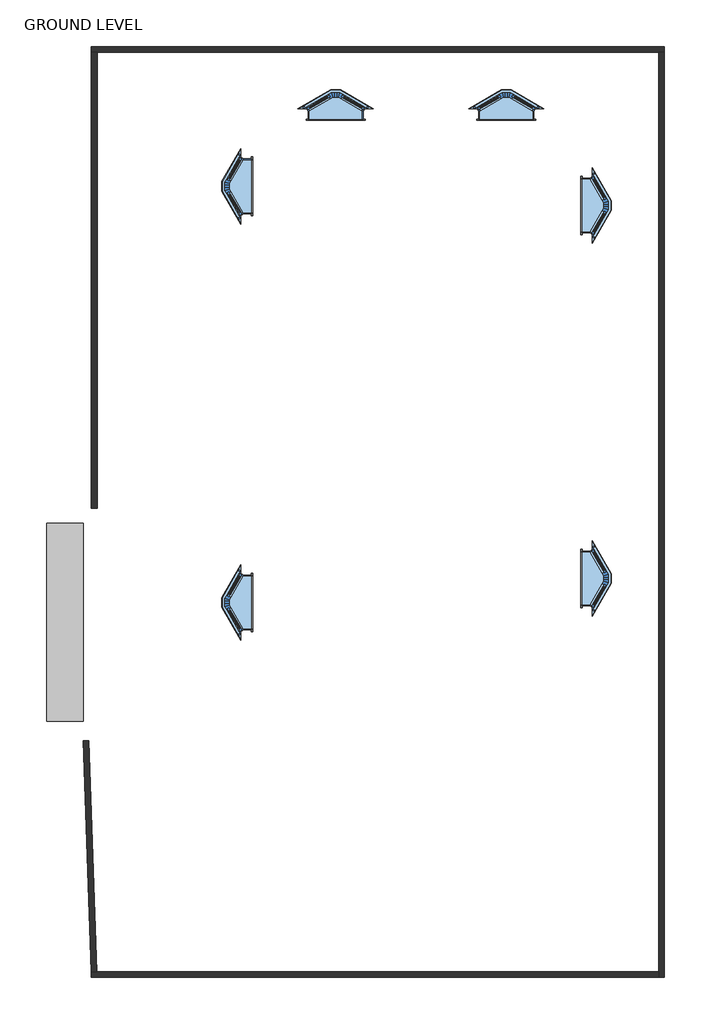
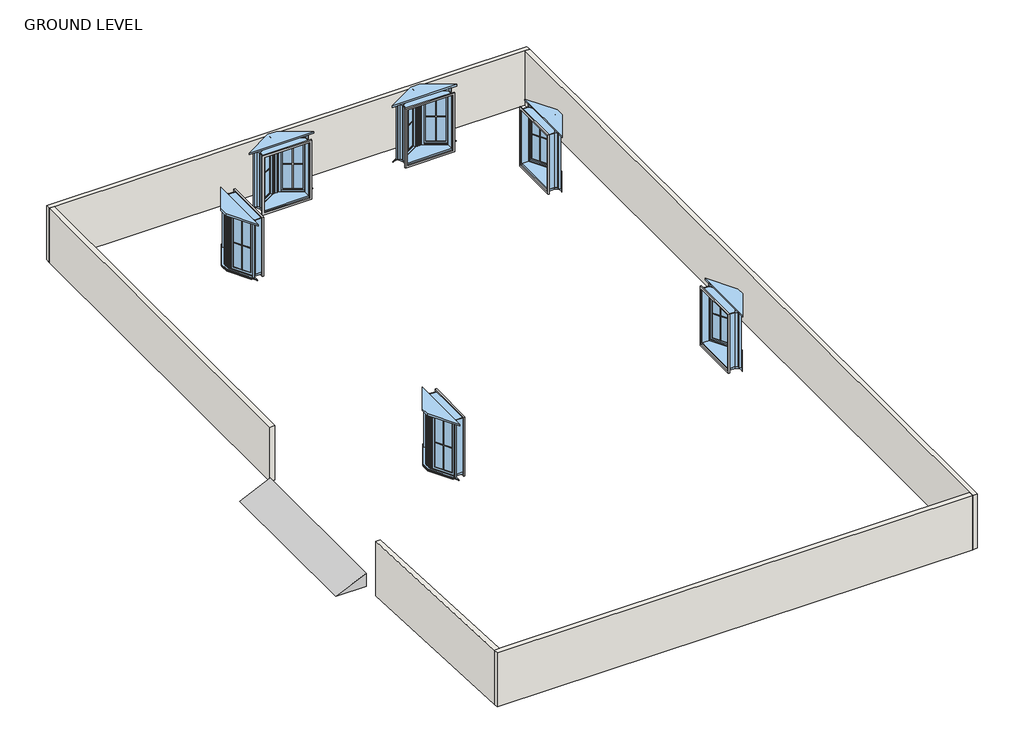
# One storey: 19 proxies, 6 windows, 5 walls.
"""IFC4 building model written with IfcOpenShell, lengths in millimetres."""

from ifc_helpers import new_model, si_unit, origin, origin_with_axes, place, context, project, spatial, polyline, outline, extrude, faceted_brep, transform, mapped, element, save
from components import generic_models_2_generic_models_2_939c1542, muntin_pattern_2x2_muntin_pattern_2x2_75bf01dd, muntin_pattern_2x2_muntin_pattern_2x2_32baafd4, trim_window_interior_flat_picture_frame_1060724f, window_bay_casement_30_degree_angle_30_angle_window_doors_2_b97d1700

model = new_model("IFC4")

# Units and contexts
model_context = context("Model", 3, world=origin())
ifc_project = project(units=[si_unit("LENGTHUNIT", "METRE", prefix="MILLI")], contexts=[model_context])

# Site, building, storey
site = spatial("IfcSite", under=ifc_project)
building = spatial("IfcBuilding", under=site)
storey = spatial("IfcBuildingStorey", under=building, Name="GROUND LEVEL", Elevation=0.0)

# Proxies
placement = place(None, origin())
generic_models_2_generic_models_2_shape = generic_models_2_generic_models_2_939c1542(model_context)
element("IfcBuildingElementProxy", 1, Name="Generic Models 2 : Generic Models 2", ObjectType="Generic Models 2 : Generic Models 2", at=placement, inside=storey, context=model_context, shape_type="MappedRepresentation", body=[
    mapped(generic_models_2_generic_models_2_shape, transform((0.0, 0.0, 0.0), x_axis=(1.0, 0.0, 0.0), y_axis=(0.0, 1.0, 0.0), z_axis=(0.0, 0.0, 1.0))),
])
muntin_pattern_2x2_muntin_pattern_2x2_shape = muntin_pattern_2x2_muntin_pattern_2x2_75bf01dd(model_context)
element("IfcBuildingElementProxy", 2, Name="Muntin Pattern_2x2 : Muntin Pattern_2x2", ObjectType="Muntin Pattern_2x2 : Muntin Pattern_2x2", at=placement, inside=storey, context=model_context, shape_type="MappedRepresentation", body=[
    mapped(muntin_pattern_2x2_muntin_pattern_2x2_shape, transform((-17494.1197687, 9500.6003691, 730.25), x_axis=(-0.49999999999999245, 0.866025403784443, 0.0), y_axis=(-0.866025403784443, -0.49999999999999245, 0.0), z_axis=(0.0, 0.0, 1.0))),
])
element("IfcBuildingElementProxy", 3, Name="Muntin Pattern_2x2 : Muntin Pattern_2x2", ObjectType="Muntin Pattern_2x2 : Muntin Pattern_2x2", at=placement, inside=storey, context=model_context, shape_type="MappedRepresentation", body=[
    mapped(muntin_pattern_2x2_muntin_pattern_2x2_shape, transform((-15626.2408789, 11750.0736953, 730.25), x_axis=(0.8660254037844439, 0.49999999999999095, 0.0), y_axis=(-0.49999999999999095, 0.8660254037844439, 0.0), z_axis=(0.0, 0.0, 1.0))),
])
element("IfcBuildingElementProxy", 4, Name="Muntin Pattern_2x2 : Muntin Pattern_2x2", ObjectType="Muntin Pattern_2x2 : Muntin Pattern_2x2", at=placement, inside=storey, context=model_context, shape_type="MappedRepresentation", body=[
    mapped(muntin_pattern_2x2_muntin_pattern_2x2_shape, transform((-11828.9408789, 11750.0736953, 730.25), x_axis=(0.8660254037844439, 0.49999999999999095, 0.0), y_axis=(-0.49999999999999095, 0.8660254037844439, 0.0), z_axis=(0.0, 0.0, 1.0))),
])
element("IfcBuildingElementProxy", 5, Name="Muntin Pattern_2x2 : Muntin Pattern_2x2", ObjectType="Muntin Pattern_2x2 : Muntin Pattern_2x2", at=placement, inside=storey, context=model_context, shape_type="MappedRepresentation", body=[
    mapped(muntin_pattern_2x2_muntin_pattern_2x2_shape, transform((-9388.9675526, 9837.7448055, 730.25), x_axis=(0.4999999999999924, -0.866025403784443, 0.0), y_axis=(0.866025403784443, 0.4999999999999924, 0.0), z_axis=(0.0, 0.0, 1.0))),
])
element("IfcBuildingElementProxy", 6, Name="Muntin Pattern_2x2 : Muntin Pattern_2x2", ObjectType="Muntin Pattern_2x2 : Muntin Pattern_2x2", at=placement, inside=storey, context=model_context, shape_type="MappedRepresentation", body=[
    mapped(muntin_pattern_2x2_muntin_pattern_2x2_shape, transform((-9388.9675526, 1538.2948055, 730.25), x_axis=(0.4999999999999924, -0.866025403784443, 0.0), y_axis=(0.866025403784443, 0.4999999999999924, 0.0), z_axis=(0.0, 0.0, 1.0))),
])
element("IfcBuildingElementProxy", 7, Name="Muntin Pattern_2x2 : Muntin Pattern_2x2", ObjectType="Muntin Pattern_2x2 : Muntin Pattern_2x2", at=placement, inside=storey, context=model_context, shape_type="MappedRepresentation", body=[
    mapped(muntin_pattern_2x2_muntin_pattern_2x2_shape, transform((-17494.1197687, 242.3003691, 730.25), x_axis=(-0.49999999999999245, 0.866025403784443, 0.0), y_axis=(-0.866025403784443, -0.49999999999999245, 0.0), z_axis=(0.0, 0.0, 1.0))),
])
muntin_pattern_2x2_muntin_pattern_2x2_2_shape = muntin_pattern_2x2_muntin_pattern_2x2_32baafd4(model_context)
element("IfcBuildingElementProxy", 8, Name="Muntin Pattern_2x2 : Muntin Pattern_2x2", ObjectType="Muntin Pattern_2x2 : Muntin Pattern_2x2", at=placement, inside=storey, context=model_context, shape_type="MappedRepresentation", body=[
    mapped(muntin_pattern_2x2_muntin_pattern_2x2_2_shape, transform((-17494.1197687, 10263.1948055, 730.25), x_axis=(-0.4999999999999952, -0.8660254037844415, 0.0), y_axis=(0.8660254037844415, -0.4999999999999952, 0.0), z_axis=(0.0, 0.0, 1.0))),
])
element("IfcBuildingElementProxy", 9, Name="Muntin Pattern_2x2 : Muntin Pattern_2x2", ObjectType="Muntin Pattern_2x2 : Muntin Pattern_2x2", at=placement, inside=storey, context=model_context, shape_type="MappedRepresentation", body=[
    mapped(muntin_pattern_2x2_muntin_pattern_2x2_2_shape, transform((-14863.6464424, 11750.0736953, 730.25), x_axis=(-0.8660254037844406, 0.4999999999999967, 0.0), y_axis=(-0.4999999999999967, -0.8660254037844406, 0.0), z_axis=(0.0, 0.0, 1.0))),
])
element("IfcBuildingElementProxy", 10, Name="Muntin Pattern_2x2 : Muntin Pattern_2x2", ObjectType="Muntin Pattern_2x2 : Muntin Pattern_2x2", at=placement, inside=storey, context=model_context, shape_type="MappedRepresentation", body=[
    mapped(muntin_pattern_2x2_muntin_pattern_2x2_2_shape, transform((-11066.3464424, 11750.0736953, 730.25), x_axis=(-0.8660254037844406, 0.4999999999999967, 0.0), y_axis=(-0.4999999999999967, -0.8660254037844406, 0.0), z_axis=(0.0, 0.0, 1.0))),
])
element("IfcBuildingElementProxy", 11, Name="Muntin Pattern_2x2 : Muntin Pattern_2x2", ObjectType="Muntin Pattern_2x2 : Muntin Pattern_2x2", at=placement, inside=storey, context=model_context, shape_type="MappedRepresentation", body=[
    mapped(muntin_pattern_2x2_muntin_pattern_2x2_2_shape, transform((-9388.9675526, 9075.1503691, 730.25), x_axis=(0.4999999999999953, 0.8660254037844415, 0.0), y_axis=(-0.8660254037844415, 0.4999999999999953, 0.0), z_axis=(0.0, 0.0, 1.0))),
])
element("IfcBuildingElementProxy", 12, Name="Muntin Pattern_2x2 : Muntin Pattern_2x2", ObjectType="Muntin Pattern_2x2 : Muntin Pattern_2x2", at=placement, inside=storey, context=model_context, shape_type="MappedRepresentation", body=[
    mapped(muntin_pattern_2x2_muntin_pattern_2x2_2_shape, transform((-9388.9675526, 775.7003691, 730.25), x_axis=(0.4999999999999953, 0.8660254037844415, 0.0), y_axis=(-0.8660254037844415, 0.4999999999999953, 0.0), z_axis=(0.0, 0.0, 1.0))),
])
element("IfcBuildingElementProxy", 13, Name="Muntin Pattern_2x2 : Muntin Pattern_2x2", ObjectType="Muntin Pattern_2x2 : Muntin Pattern_2x2", at=placement, inside=storey, context=model_context, shape_type="MappedRepresentation", body=[
    mapped(muntin_pattern_2x2_muntin_pattern_2x2_2_shape, transform((-17494.1197687, 1004.8948055, 730.25), x_axis=(-0.4999999999999952, -0.8660254037844415, 0.0), y_axis=(0.8660254037844415, -0.4999999999999952, 0.0), z_axis=(0.0, 0.0, 1.0))),
])
trim_window_interior_flat_picture_frame_shape = trim_window_interior_flat_picture_frame_1060724f(model_context)
element("IfcBuildingElementProxy", 14, Name="Trim-Window-Interior-Flat : Picture Frame", ObjectType="Trim-Window-Interior-Flat : Picture Frame", at=placement, inside=storey, context=model_context, shape_type="MappedRepresentation", body=[
    mapped(trim_window_interior_flat_picture_frame_shape, transform((-17124.5436606, 9881.8975873, 2184.4), x_axis=(0.0, 1.0, 0.0), y_axis=(0.0, 0.0, 1.0), z_axis=(1.0, 0.0, 0.0))),
])
element("IfcBuildingElementProxy", 15, Name="Trim-Window-Interior-Flat : Picture Frame", ObjectType="Trim-Window-Interior-Flat : Picture Frame", at=placement, inside=storey, context=model_context, shape_type="MappedRepresentation", body=[
    mapped(trim_window_interior_flat_picture_frame_shape, transform((-15244.9436606, 11380.4975873, 2184.4), x_axis=(1.0, 0.0, 0.0), y_axis=(0.0, 0.0, 1.0), z_axis=(0.0, -1.0, 0.0))),
])
element("IfcBuildingElementProxy", 16, Name="Trim-Window-Interior-Flat : Picture Frame", ObjectType="Trim-Window-Interior-Flat : Picture Frame", at=placement, inside=storey, context=model_context, shape_type="MappedRepresentation", body=[
    mapped(trim_window_interior_flat_picture_frame_shape, transform((-11447.6436606, 11380.4975873, 2184.4), x_axis=(1.0, 0.0, 0.0), y_axis=(0.0, 0.0, 1.0), z_axis=(0.0, -1.0, 0.0))),
])
element("IfcBuildingElementProxy", 17, Name="Trim-Window-Interior-Flat : Picture Frame", ObjectType="Trim-Window-Interior-Flat : Picture Frame", at=placement, inside=storey, context=model_context, shape_type="MappedRepresentation", body=[
    mapped(trim_window_interior_flat_picture_frame_shape, transform((-9758.5436606, 9456.4475873, 2184.4), x_axis=(0.0, -1.0, 0.0), y_axis=(0.0, 0.0, 1.0), z_axis=(-1.0, 0.0, 0.0))),
])
element("IfcBuildingElementProxy", 18, Name="Trim-Window-Interior-Flat : Picture Frame", ObjectType="Trim-Window-Interior-Flat : Picture Frame", at=placement, inside=storey, context=model_context, shape_type="MappedRepresentation", body=[
    mapped(trim_window_interior_flat_picture_frame_shape, transform((-9758.5436606, 1156.9975873, 2184.4), x_axis=(0.0, -1.0, 0.0), y_axis=(0.0, 0.0, 1.0), z_axis=(-1.0, 0.0, 0.0))),
])
element("IfcBuildingElementProxy", 19, Name="Trim-Window-Interior-Flat : Picture Frame", ObjectType="Trim-Window-Interior-Flat : Picture Frame", at=placement, inside=storey, context=model_context, shape_type="MappedRepresentation", body=[
    mapped(trim_window_interior_flat_picture_frame_shape, transform((-17124.5436606, 623.5975873, 2184.4), x_axis=(0.0, 1.0, 0.0), y_axis=(0.0, 0.0, 1.0), z_axis=(1.0, 0.0, 0.0))),
])

# Walls
element("IfcWall", 20, ObjectType="outer wall 5\"", at=placement, inside=storey, context=model_context, shape_type="Brep", body=[
    faceted_brep([(-8056.7436606, -7593.3024127, 0.0), (-20555.7611295, -7593.3024127, 0.0), (-20682.8385416, -7593.3024127, 0.0), (-20682.8385416, -7593.3024127, 1524.0), (-20555.7611295, -7593.3024127, 1524.0), (-8056.7436606, -7593.3024127, 1524.0), (-8056.7436606, -7720.3024127, 0.0), (-8056.7436606, -7720.3024127, 1524.0), (-20678.4036039, -7720.3024127, 1524.0), (-20678.4036039, -7720.3024127, 0.0)], [[[0, 1, 2, 3, 4, 5]], [[6, 7, 8, 9]], [[2, 1, 0, 6, 9]], [[5, 4, 3, 8, 7]], [[3, 2, 9, 8]], [[0, 5, 7, 6]]]),
])
element("IfcWall", 21, ObjectType="outer wall 5\"", at=placement, inside=storey, context=model_context, shape_type="SweptSolid", body=[
    extrude(outline(polyline([(-20735.26534, -2452.9743764), (-20555.7611295, -7593.3024127), (-20682.8385416, -7593.3024127), (-20862.187975, -2457.4066125), (-20735.26534, -2452.9743764)])), origin_with_axes(), (0.0, 0.0, 1.0), 1524.0),
])
element("IfcWall", 22, ObjectType="outer wall 5\"", at=placement, inside=storey, context=model_context, shape_type="SweptSolid", body=[
    extrude(outline(polyline([(-20680.5436606, 2724.3746859), (-20680.5436606, 12866.3975873), (-20553.5436606, 12866.3975873), (-20553.5436606, 2724.3746859), (-20680.5436606, 2724.3746859)])), origin_with_axes(), (0.0, 0.0, 1.0), 1524.0),
])
element("IfcWall", 23, ObjectType="outer wall 5\"", at=placement, inside=storey, context=model_context, shape_type="Brep", body=[
    faceted_brep([(-20680.5436606, 12866.3975873, 0.0), (-20553.5436606, 12866.3975873, 0.0), (-8056.7436606, 12866.3975873, 0.0), (-7929.7436606, 12866.3975873, 0.0), (-7929.7436606, 12866.3975873, 1524.0), (-8056.7436606, 12866.3975873, 1524.0), (-20553.5436606, 12866.3975873, 1524.0), (-20680.5436606, 12866.3975873, 1524.0), (-20680.5436606, 12993.3975873, 0.0), (-20680.5436606, 12993.3975873, 1524.0), (-7929.7436606, 12993.3975873, 1524.0), (-7929.7436606, 12993.3975873, 0.0)], [[[0, 1, 2, 3, 4, 5, 6, 7]], [[8, 9, 10, 11]], [[3, 2, 1, 0, 8, 11]], [[7, 6, 5, 4, 10, 9]], [[4, 3, 11, 10]], [[0, 7, 9, 8]]]),
])
element("IfcWall", 24, ObjectType="outer wall 5\"", at=placement, inside=storey, context=model_context, shape_type="Brep", body=[
    faceted_brep([(-8056.7436606, 12866.3975873, 0.0), (-8056.7436606, -7593.3024127, 0.0), (-8056.7436606, -7720.3024127, 0.0), (-8056.7436606, -7720.3024127, 1524.0), (-8056.7436606, -7593.3024127, 1524.0), (-8056.7436606, 12866.3975873, 1524.0), (-7929.7436606, 12866.3975873, 0.0), (-7929.7436606, 12866.3975873, 1524.0), (-7929.7436606, -7720.3024127, 1524.0), (-7929.7436606, -7720.3024127, 0.0)], [[[0, 1, 2, 3, 4, 5]], [[6, 7, 8, 9]], [[2, 1, 0, 6, 9]], [[5, 4, 3, 8, 7]], [[0, 5, 7, 6]], [[3, 2, 9, 8]]]),
])

# Windows
window_bay_casement_30_degree_angle_30_angle_window_doors_2_shape = window_bay_casement_30_degree_angle_30_angle_window_doors_2_b97d1700(model_context)
element("IfcWindow", 25, ObjectType="Window-Bay-Casement-30_Degree_Angle : 30 ANGLE WINDOW DOORS", at=placement, inside=storey, context=model_context, shape_type="MappedRepresentation", body=[
    mapped(window_bay_casement_30_degree_angle_30_angle_window_doors_2_shape, transform((-15244.9436606, 11494.7975873, 0.0), x_axis=(1.0, 0.0, 0.0), y_axis=(0.0, 1.0, 0.0), z_axis=(0.0, 0.0, 1.0))),
])
element("IfcWindow", 26, ObjectType="Window-Bay-Casement-30_Degree_Angle : 30 ANGLE WINDOW DOORS", at=placement, inside=storey, context=model_context, shape_type="MappedRepresentation", body=[
    mapped(window_bay_casement_30_degree_angle_30_angle_window_doors_2_shape, transform((-11447.6436606, 11494.7975873, 0.0), x_axis=(1.0, 0.0, 0.0), y_axis=(0.0, 1.0, 0.0), z_axis=(0.0, 0.0, 1.0))),
])
element("IfcWindow", 27, ObjectType="Window-Bay-Casement-30_Degree_Angle : 30 ANGLE WINDOW DOORS", at=placement, inside=storey, context=model_context, shape_type="MappedRepresentation", body=[
    mapped(window_bay_casement_30_degree_angle_30_angle_window_doors_2_shape, transform((-9644.2436606, 9456.4475873, 0.0), x_axis=(0.0, -1.0, 0.0), y_axis=(1.0, 0.0, 0.0), z_axis=(0.0, 0.0, 1.0))),
])
element("IfcWindow", 28, ObjectType="Window-Bay-Casement-30_Degree_Angle : 30 ANGLE WINDOW DOORS", at=placement, inside=storey, context=model_context, shape_type="MappedRepresentation", body=[
    mapped(window_bay_casement_30_degree_angle_30_angle_window_doors_2_shape, transform((-9644.2436606, 1156.9975873, 0.0), x_axis=(0.0, -1.0, 0.0), y_axis=(1.0, 0.0, 0.0), z_axis=(0.0, 0.0, 1.0))),
])
element("IfcWindow", 29, ObjectType="Window-Bay-Casement-30_Degree_Angle : 30 ANGLE WINDOW DOORS", at=placement, inside=storey, context=model_context, shape_type="MappedRepresentation", body=[
    mapped(window_bay_casement_30_degree_angle_30_angle_window_doors_2_shape, transform((-17238.8436606, 623.5975873, 0.0), x_axis=(0.0, 1.0, 0.0), y_axis=(-1.0, 0.0, 0.0), z_axis=(0.0, 0.0, 1.0))),
])
element("IfcWindow", 30, ObjectType="Window-Bay-Casement-30_Degree_Angle : 30 ANGLE WINDOW DOORS 3", at=placement, inside=storey, context=model_context, shape_type="MappedRepresentation", body=[
    mapped(window_bay_casement_30_degree_angle_30_angle_window_doors_2_shape, transform((-17238.8436606, 9881.8975873, 0.0), x_axis=(0.0, 1.0, 0.0), y_axis=(-1.0, 0.0, 0.0), z_axis=(0.0, 0.0, 1.0))),
])

save(model, "model.ifc")

# Revit data of these elements
# Type "Muntin Pattern_2x2 : Muntin Pattern_2x2"
#   Width [instance default] = 4' - 0"
#   Thickness = 0' - 0 1/2"
#   Height [instance default] = 4' - 0"
#   Distance = 0' - 0 3/4"
#   Interior Material [instance default] = none
#   Exterior Material [instance default] = none
#   Default Elevation = 0
# Type "Trim-Window-Interior-Flat : Picture Frame"
#   Trim Thickness_Picture Frame = 0' - 1 1/4"
#   Trim Width = 0' - 2 1/4"
#   Trim Thickness_with Sill = 0' - 0 3/4"
#   Sill Thickness = 0' - 1 1/4"
#   Opening Width [instance default] = 2' - 0"
#   Opening Height [instance default] = 3' - 0"
#   Default Elevation = 4' - 0"
#   Sill = no
#   Picture Frame = yes
#   Trim Material [instance default] = none
# Type "outer wall 5\""
#   Assembly Code = "B2010"
#   Layers, outside or top first: 0' - 5" "BROWN" (function 1)
# Type "Window-Bay-Casement-30_Degree_Angle : 30 ANGLE WINDOW DOORS"
#   Type Mark = "19"
#   Fire Rating = "0.5h"
#   Assembly Code = "B2020100"
#   Analytic Construction = "Double glazing - domestic"
#   Width of Middle Sash = 0' - 2.5827"
#   Width = 4' - 0"
#   Visual Light Transmittance = 0.81
#   Thermal Resistance (R) = 1.8146 (h·ft²·°F)/BTU
#   Solar Heat Gain Coefficient = 0.76
#   Rough Width = 4' - 0 1/2"
#   Rough Height = 5' - 0 1/2"
#   Length 2 = 0' - 7.25458"
#   Length 1 = 1' - 8.70865"
#   Wall Thickness [instance default] = 0' - 6"
#   Trim Width = 4' - 4 43/64"
#   Trim Height = 5' - 0"
#   Height 1 = 5' - 2"
#   Height = 5' - 0"
#   Heat Transfer Coefficient (U) = 0.5511 BTU/(h·ft²·°F)
#   Depth = 1' - 2"
#   Default Sill Height = 2' - 0"
#   Angle = 30.00°
#   Muntin Visibility = yes
#   Interior Trim Visibility [instance default] = yes
#   Exterior Trim Visibility [instance default] = yes
#   Muntin Pattern = Muntin Pattern_2x2 : Muntin Pattern_2x2
#   Interior Trim Material = Wood - Stained
#   Exterior Trim Material = Clad - White
#   Exterior Trim = element 398720
#   Interior Trim = Trim-Window-Interior-Flat : Picture Frame
#   Interior Frame Material = Wood - Stained
#   Glass Panel Material = Glass
#   Exterior Frame Material = Clad - White
#   Wall Closure = (empty or 0)
# Type "Window-Bay-Casement-30_Degree_Angle : 30 ANGLE WINDOW DOORS 3"
#   Type Mark = "21"
#   Fire Rating = "0.5h"
#   Assembly Code = "B2020100"
#   Analytic Construction = "Double glazing - domestic"
#   Width of Middle Sash = 0' - 2.5827"
#   Width = 4' - 0"
#   Visual Light Transmittance = 0.81
#   Thermal Resistance (R) = 1.8146 (h·ft²·°F)/BTU
#   Solar Heat Gain Coefficient = 0.76
#   Rough Width = 4' - 0 1/2"
#   Rough Height = 5' - 0 1/2"
#   Length 2 = 0' - 7.25458"
#   Length 1 = 1' - 8.70865"
#   Wall Thickness [instance default] = 0' - 6"
#   Trim Width = 4' - 4 43/64"
#   Trim Height = 5' - 0"
#   Height 1 = 5' - 2"
#   Height = 5' - 0"
#   Heat Transfer Coefficient (U) = 0.5511 BTU/(h·ft²·°F)
#   Depth = 1' - 2"
#   Default Sill Height = 2' - 0"
#   Angle = 30.00°
#   Muntin Visibility = yes
#   Interior Trim Visibility [instance default] = yes
#   Exterior Trim Visibility [instance default] = yes
#   Muntin Pattern = Muntin Pattern_2x2 : Muntin Pattern_2x2
#   Interior Trim Material = Wood - Stained
#   Exterior Trim Material = Clad - White
#   Exterior Trim = element 398720
#   Interior Trim = Trim-Window-Interior-Flat : Picture Frame
#   Interior Frame Material = Wood - Stained
#   Glass Panel Material = Glass
#   Exterior Frame Material = Clad - White
#   Wall Closure = (empty or 0)
# Element 1 (IfcBuildingElementProxy, "Generic Models 2 : Generic Models 2")
#   Phase Created = New Construction
#   Materials on its faces: "Default New Material(1)"
# Elements 2, 3, 4, 5, 6, 7, 8, 9, 10, 11, 12, 13 (IfcBuildingElementProxy, "Muntin Pattern_2x2 : Muntin Pattern_2x2")
#   Width = 1' - 6"
#   Height = 4' - 6 1/2"
#   Interior Material = Wood - Stained
#   Exterior Material = Clad - White
#   Phase Created = New Construction
#   Materials on its faces: "Clad - White", "Wood - Stained"
# Elements 14, 15, 16, 17, 18, 19 (IfcBuildingElementProxy, "Trim-Window-Interior-Flat : Picture Frame")
#   Opening Width = 4' - 0"
#   Opening Height = 5' - 2"
#   Trim Material = Wood - Stained
#   Phase Created = New Construction
#   Materials on its faces: "Wood - Stained"
# Elements 20, 21, 22, 23, 24 (IfcWall, "outer wall 5\"")
#   Top Offset = 0' - 0"
#   Base Offset = 0' - 0"
#   Unconnected Height = 5' - 0"
#   wall height = 5' - 0"
#   Phase Created = New Construction
#   Base Constraint = GROUND LEVEL
#   Materials on its faces: "BROWN"
# Element 25 (IfcWindow, "Window-Bay-Casement-30_Degree_Angle : 30 ANGLE WINDOW DOORS")
#   Mark = "3"
#   Interior Trim Visibility = yes
#   Exterior Trim Visibility = yes
#   Phase Created = New Construction
#   Materials on its faces: "Clad - White", "Wood - Stained", "Glass"
# Element 26 (IfcWindow, "Window-Bay-Casement-30_Degree_Angle : 30 ANGLE WINDOW DOORS")
#   Mark = "4"
#   Interior Trim Visibility = yes
#   Exterior Trim Visibility = yes
#   Phase Created = New Construction
#   Materials on its faces: "Clad - White", "Wood - Stained", "Glass"
# Element 27 (IfcWindow, "Window-Bay-Casement-30_Degree_Angle : 30 ANGLE WINDOW DOORS")
#   Mark = "5"
#   Interior Trim Visibility = yes
#   Exterior Trim Visibility = yes
#   Phase Created = New Construction
#   Materials on its faces: "Clad - White", "Wood - Stained", "Glass"
# Element 28 (IfcWindow, "Window-Bay-Casement-30_Degree_Angle : 30 ANGLE WINDOW DOORS")
#   Mark = "6"
#   Interior Trim Visibility = yes
#   Exterior Trim Visibility = yes
#   Phase Created = New Construction
#   Materials on its faces: "Clad - White", "Wood - Stained", "Glass"
# Element 29 (IfcWindow, "Window-Bay-Casement-30_Degree_Angle : 30 ANGLE WINDOW DOORS")
#   Mark = "7"
#   Interior Trim Visibility = yes
#   Exterior Trim Visibility = yes
#   Phase Created = New Construction
#   Materials on its faces: "Clad - White", "Wood - Stained", "Glass"
# Element 30 (IfcWindow, "Window-Bay-Casement-30_Degree_Angle : 30 ANGLE WINDOW DOORS 3")
#   Mark = "2"
#   Interior Trim Visibility = yes
#   Exterior Trim Visibility = yes
#   Phase Created = New Construction
#   Materials on its faces: "Clad - White", "Wood - Stained", "Glass"
# Materials
#   "BROWN": class "Generic", colour RGB 120 120 120, transparency 0, Cost = 0
#   "Wood - Stained": class "Wood", colour RGB 224 178 126, transparency 0, Cost = 0
#   "Clad - White": class "Wood", colour RGB 30 30 30, transparency 0, Cost = 0
#   "Glass": class "Glass", colour RGB 0 128 192, transparency 0.75, Description = "Soda Lime Glass", Cost = 0
#   "Default New Material(1)": class "Generic", colour RGB 120 120 120, transparency 0, Cost = 0
